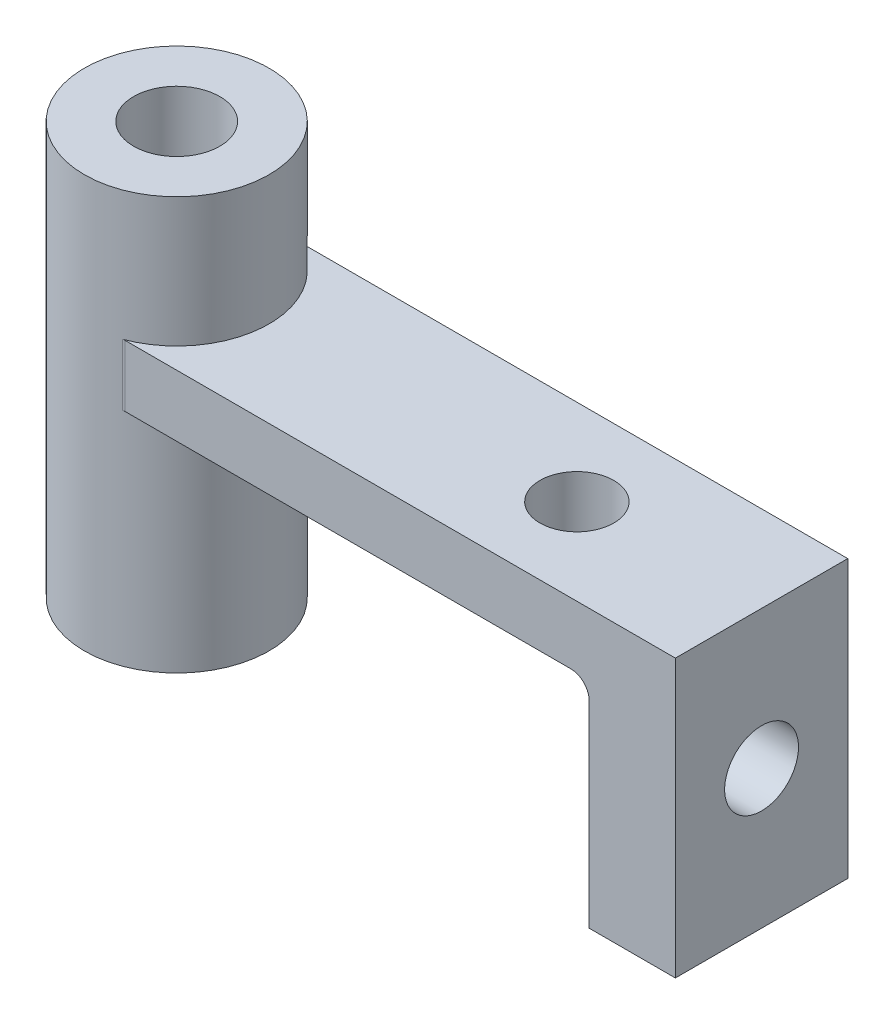
ISO-10303-21;
HEADER;
FILE_DESCRIPTION(('STEP AP214'),'2;1');
FILE_NAME('part.step','',(''),(''),'','','');
FILE_SCHEMA(('AUTOMOTIVE_DESIGN { 1 0 10303 214 1 1 1 1 }'));
ENDSEC;
DATA;
#1=APPLICATION_CONTEXT('core data for automotive mechanical design processes');
#2=APPLICATION_PROTOCOL_DEFINITION('international standard','automotive_design',2000,#1);
#3=PRODUCT_CONTEXT('',#1,'mechanical');
#4=PRODUCT('Part','Part','',(#3));
#5=PRODUCT_RELATED_PRODUCT_CATEGORY('part','',(#4));
#6=PRODUCT_DEFINITION_FORMATION('','',#4);
#7=PRODUCT_DEFINITION_CONTEXT('part definition',#1,'design');
#8=PRODUCT_DEFINITION('design','',#6,#7);
#9=PRODUCT_DEFINITION_SHAPE('','',#8);
#10=(LENGTH_UNIT() NAMED_UNIT(*) SI_UNIT(.MILLI.,.METRE.));
#11=(NAMED_UNIT(*) PLANE_ANGLE_UNIT() SI_UNIT($,.RADIAN.));
#12=(NAMED_UNIT(*) SI_UNIT($,.STERADIAN.) SOLID_ANGLE_UNIT());
#13=UNCERTAINTY_MEASURE_WITH_UNIT(LENGTH_MEASURE(1.E-05),#10,'distance_accuracy_value','');
#14=(GEOMETRIC_REPRESENTATION_CONTEXT(3) GLOBAL_UNCERTAINTY_ASSIGNED_CONTEXT((#13)) GLOBAL_UNIT_ASSIGNED_CONTEXT((#10,
#11,#12)) REPRESENTATION_CONTEXT('',''));
#15=CARTESIAN_POINT('',(0.,0.,0.));
#16=DIRECTION('',(0.,0.,1.));
#17=DIRECTION('',(1.,0.,0.));
#18=AXIS2_PLACEMENT_3D('',#15,#16,#17);
#19=CARTESIAN_POINT('',(78.,-3.,28.));
#20=DIRECTION('',(0.,0.,-1.));
#21=DIRECTION('',(-1.,0.,0.));
#22=AXIS2_PLACEMENT_3D('',#19,#20,#21);
#23=PLANE('',#22);
#24=DIRECTION('',(-1.,0.,0.));
#25=VECTOR('',#24,1.);
#26=CARTESIAN_POINT('',(95.,9.99999999999999,28.));
#27=LINE('',#26,#25);
#28=CARTESIAN_POINT('',(95.,9.99999999999999,28.));
#29=VERTEX_POINT('',#28);
#30=CARTESIAN_POINT('',(5.56776436283002,9.99999999999999,28.));
#31=VERTEX_POINT('',#30);
#32=EDGE_CURVE('E145',#29,#31,#27,.T.);
#33=ORIENTED_EDGE('',*,*,#32,.T.);
#34=DIRECTION('',(0.,1.,0.));
#35=VECTOR('',#34,1.);
#36=CARTESIAN_POINT('',(5.56776436283002,0.,28.));
#37=LINE('',#36,#35);
#38=CARTESIAN_POINT('',(5.56776436283002,0.,28.));
#39=VERTEX_POINT('',#38);
#40=EDGE_CURVE('E63',#31,#39,#37,.F.);
#41=ORIENTED_EDGE('',*,*,#40,.T.);
#42=DIRECTION('',(1.,0.,0.));
#43=VECTOR('',#42,1.);
#44=CARTESIAN_POINT('',(0.,0.,28.));
#45=LINE('',#44,#43);
#46=CARTESIAN_POINT('',(78.,0.,28.));
#47=VERTEX_POINT('',#46);
#48=EDGE_CURVE('E111',#39,#47,#45,.T.);
#49=ORIENTED_EDGE('',*,*,#48,.T.);
#50=CARTESIAN_POINT('',(78.,-3.,28.));
#51=DIRECTION('',(0.,0.,-1.));
#52=DIRECTION('',(-1.,0.,0.));
#53=AXIS2_PLACEMENT_3D('',#50,#51,#52);
#54=CIRCLE('',#53,3.);
#55=CARTESIAN_POINT('',(81.,-3.00000000000002,28.));
#56=VERTEX_POINT('',#55);
#57=EDGE_CURVE('E112',#47,#56,#54,.T.);
#58=ORIENTED_EDGE('',*,*,#57,.T.);
#59=DIRECTION('',(0.,-1.,0.));
#60=VECTOR('',#59,1.);
#61=CARTESIAN_POINT('',(81.,-3.00000000000002,28.));
#62=LINE('',#61,#60);
#63=CARTESIAN_POINT('',(81.,-35.,28.));
#64=VERTEX_POINT('',#63);
#65=EDGE_CURVE('E135',#56,#64,#62,.T.);
#66=ORIENTED_EDGE('',*,*,#65,.T.);
#67=DIRECTION('',(1.,0.,0.));
#68=VECTOR('',#67,1.);
#69=CARTESIAN_POINT('',(81.,-35.,28.));
#70=LINE('',#69,#68);
#71=CARTESIAN_POINT('',(95.,-35.,28.));
#72=VERTEX_POINT('',#71);
#73=EDGE_CURVE('E132',#64,#72,#70,.T.);
#74=ORIENTED_EDGE('',*,*,#73,.T.);
#75=DIRECTION('',(0.,1.,0.));
#76=VECTOR('',#75,1.);
#77=CARTESIAN_POINT('',(95.,-35.,28.));
#78=LINE('',#77,#76);
#79=EDGE_CURVE('E140',#72,#29,#78,.T.);
#80=ORIENTED_EDGE('',*,*,#79,.T.);
#81=EDGE_LOOP('',(#33,#41,#49,#58,#66,#74,#80));
#82=FACE_BOUND('',#81,.T.);
#83=ADVANCED_FACE('F43',(#82),#23,.F.);
#84=CARTESIAN_POINT('',(78.,-3.,0.));
#85=DIRECTION('',(0.,0.,-1.));
#86=DIRECTION('',(-1.,0.,0.));
#87=AXIS2_PLACEMENT_3D('',#84,#85,#86);
#88=PLANE('',#87);
#89=DIRECTION('',(1.,0.,0.));
#90=VECTOR('',#89,1.);
#91=CARTESIAN_POINT('',(0.,0.,0.));
#92=LINE('',#91,#90);
#93=CARTESIAN_POINT('',(5.56776436283002,0.,0.));
#94=VERTEX_POINT('',#93);
#95=CARTESIAN_POINT('',(78.,0.,0.));
#96=VERTEX_POINT('',#95);
#97=EDGE_CURVE('E121',#94,#96,#92,.T.);
#98=ORIENTED_EDGE('',*,*,#97,.F.);
#99=DIRECTION('',(0.,-1.,0.));
#100=VECTOR('',#99,1.);
#101=CARTESIAN_POINT('',(5.56776436283002,-3.,0.));
#102=LINE('',#101,#100);
#103=CARTESIAN_POINT('',(5.56776436283002,9.99999999999999,0.));
#104=VERTEX_POINT('',#103);
#105=EDGE_CURVE('E126',#94,#104,#102,.F.);
#106=ORIENTED_EDGE('',*,*,#105,.T.);
#107=DIRECTION('',(-1.,0.,0.));
#108=VECTOR('',#107,1.);
#109=CARTESIAN_POINT('',(95.,9.99999999999999,0.));
#110=LINE('',#109,#108);
#111=CARTESIAN_POINT('',(95.,9.99999999999999,0.));
#112=VERTEX_POINT('',#111);
#113=EDGE_CURVE('E117',#112,#104,#110,.T.);
#114=ORIENTED_EDGE('',*,*,#113,.F.);
#115=DIRECTION('',(0.,1.,0.));
#116=VECTOR('',#115,1.);
#117=CARTESIAN_POINT('',(95.,-35.,0.));
#118=LINE('',#117,#116);
#119=CARTESIAN_POINT('',(95.,-35.,0.));
#120=VERTEX_POINT('',#119);
#121=EDGE_CURVE('E155',#120,#112,#118,.T.);
#122=ORIENTED_EDGE('',*,*,#121,.F.);
#123=DIRECTION('',(1.,0.,0.));
#124=VECTOR('',#123,1.);
#125=CARTESIAN_POINT('',(81.,-35.,0.));
#126=LINE('',#125,#124);
#127=CARTESIAN_POINT('',(81.,-35.,0.));
#128=VERTEX_POINT('',#127);
#129=EDGE_CURVE('E154',#128,#120,#126,.T.);
#130=ORIENTED_EDGE('',*,*,#129,.F.);
#131=DIRECTION('',(0.,-1.,0.));
#132=VECTOR('',#131,1.);
#133=CARTESIAN_POINT('',(81.,-3.00000000000002,0.));
#134=LINE('',#133,#132);
#135=CARTESIAN_POINT('',(81.,-3.00000000000002,0.));
#136=VERTEX_POINT('',#135);
#137=EDGE_CURVE('E148',#136,#128,#134,.T.);
#138=ORIENTED_EDGE('',*,*,#137,.F.);
#139=CARTESIAN_POINT('',(78.,-3.,0.));
#140=DIRECTION('',(0.,0.,-1.));
#141=DIRECTION('',(-1.,0.,0.));
#142=AXIS2_PLACEMENT_3D('',#139,#140,#141);
#143=CIRCLE('',#142,3.);
#144=EDGE_CURVE('E149',#96,#136,#143,.T.);
#145=ORIENTED_EDGE('',*,*,#144,.F.);
#146=EDGE_LOOP('',(#98,#106,#114,#122,#130,#138,#145));
#147=FACE_BOUND('',#146,.T.);
#148=ADVANCED_FACE('F183',(#147),#88,.T.);
#149=CARTESIAN_POINT('',(0.,0.,28.));
#150=DIRECTION('',(0.,1.,0.));
#151=DIRECTION('',(0.,0.,1.));
#152=AXIS2_PLACEMENT_3D('',#149,#150,#151);
#153=PLANE('',#152);
#154=CARTESIAN_POINT('',(65.,0.,14.));
#155=DIRECTION('',(0.,1.,0.));
#156=DIRECTION('',(0.,0.,1.));
#157=AXIS2_PLACEMENT_3D('',#154,#155,#156);
#158=CIRCLE('',#157,6.);
#159=CARTESIAN_POINT('',(65.,0.,20.));
#160=VERTEX_POINT('',#159);
#161=EDGE_CURVE('E221',#160,#160,#158,.T.);
#162=ORIENTED_EDGE('',*,*,#161,.T.);
#163=EDGE_LOOP('',(#162));
#164=FACE_BOUND('',#163,.T.);
#165=CARTESIAN_POINT('',(0.,0.,14.));
#166=DIRECTION('',(0.,1.,0.));
#167=DIRECTION('',(0.,0.,1.));
#168=AXIS2_PLACEMENT_3D('',#165,#166,#167);
#169=CIRCLE('',#168,15.);
#170=CARTESIAN_POINT('',(5.21977909015315,0.,-0.0624999999999983));
#171=VERTEX_POINT('',#170);
#172=CARTESIAN_POINT('',(5.21977909015314,0.,28.0625));
#173=VERTEX_POINT('',#172);
#174=EDGE_CURVE('E146',#171,#173,#169,.F.);
#175=ORIENTED_EDGE('',*,*,#174,.F.);
#176=CARTESIAN_POINT('',(5.56776436283002,0.,-0.999999999999999));
#177=DIRECTION('',(0.,1.,0.));
#178=DIRECTION('',(0.,0.,1.));
#179=AXIS2_PLACEMENT_3D('',#176,#177,#178);
#180=CIRCLE('',#179,1.);
#181=EDGE_CURVE('E178',#171,#94,#180,.T.);
#182=ORIENTED_EDGE('',*,*,#181,.T.);
#183=ORIENTED_EDGE('',*,*,#97,.T.);
#184=DIRECTION('',(0.,0.,-1.));
#185=VECTOR('',#184,1.);
#186=CARTESIAN_POINT('',(78.,0.,28.));
#187=LINE('',#186,#185);
#188=EDGE_CURVE('E122',#47,#96,#187,.T.);
#189=ORIENTED_EDGE('',*,*,#188,.F.);
#190=ORIENTED_EDGE('',*,*,#48,.F.);
#191=CARTESIAN_POINT('',(5.56776436283002,0.,29.));
#192=DIRECTION('',(0.,1.,0.));
#193=DIRECTION('',(0.,0.,1.));
#194=AXIS2_PLACEMENT_3D('',#191,#192,#193);
#195=CIRCLE('',#194,1.);
#196=EDGE_CURVE('E11',#39,#173,#195,.T.);
#197=ORIENTED_EDGE('',*,*,#196,.T.);
#198=EDGE_LOOP('',(#175,#182,#183,#189,#190,#197));
#199=FACE_BOUND('',#198,.T.);
#200=ADVANCED_FACE('F125',(#164,#199),#153,.F.);
#201=CARTESIAN_POINT('',(78.,-3.,28.));
#202=DIRECTION('',(0.,0.,-1.));
#203=DIRECTION('',(-1.,0.,0.));
#204=AXIS2_PLACEMENT_3D('',#201,#202,#203);
#205=CYLINDRICAL_SURFACE('',#204,3.);
#206=ORIENTED_EDGE('',*,*,#144,.T.);
#207=DIRECTION('',(0.,0.,-1.));
#208=VECTOR('',#207,1.);
#209=CARTESIAN_POINT('',(81.,-3.00000000000002,28.));
#210=LINE('',#209,#208);
#211=EDGE_CURVE('E130',#56,#136,#210,.T.);
#212=ORIENTED_EDGE('',*,*,#211,.F.);
#213=ORIENTED_EDGE('',*,*,#57,.F.);
#214=ORIENTED_EDGE('',*,*,#188,.T.);
#215=EDGE_LOOP('',(#206,#212,#213,#214));
#216=FACE_BOUND('',#215,.T.);
#217=ADVANCED_FACE('F127',(#216),#205,.F.);
#218=CARTESIAN_POINT('',(81.,-3.00000000000002,28.));
#219=DIRECTION('',(1.,0.,0.));
#220=DIRECTION('',(0.,0.,-1.));
#221=AXIS2_PLACEMENT_3D('',#218,#219,#220);
#222=PLANE('',#221);
#223=CARTESIAN_POINT('',(81.,-12.5,14.));
#224=DIRECTION('',(1.,0.,0.));
#225=DIRECTION('',(0.,0.,-1.));
#226=AXIS2_PLACEMENT_3D('',#223,#224,#225);
#227=CIRCLE('',#226,6.);
#228=CARTESIAN_POINT('',(81.,-12.5,8.));
#229=VERTEX_POINT('',#228);
#230=EDGE_CURVE('E227',#229,#229,#227,.T.);
#231=ORIENTED_EDGE('',*,*,#230,.T.);
#232=EDGE_LOOP('',(#231));
#233=FACE_BOUND('',#232,.T.);
#234=ORIENTED_EDGE('',*,*,#137,.T.);
#235=DIRECTION('',(0.,0.,-1.));
#236=VECTOR('',#235,1.);
#237=CARTESIAN_POINT('',(81.,-35.,28.));
#238=LINE('',#237,#236);
#239=EDGE_CURVE('E162',#64,#128,#238,.T.);
#240=ORIENTED_EDGE('',*,*,#239,.F.);
#241=ORIENTED_EDGE('',*,*,#65,.F.);
#242=ORIENTED_EDGE('',*,*,#211,.T.);
#243=EDGE_LOOP('',(#234,#240,#241,#242));
#244=FACE_BOUND('',#243,.T.);
#245=ADVANCED_FACE('F202',(#233,#244),#222,.F.);
#246=CARTESIAN_POINT('',(81.,-35.,28.));
#247=DIRECTION('',(0.,1.,0.));
#248=DIRECTION('',(0.,0.,1.));
#249=AXIS2_PLACEMENT_3D('',#246,#247,#248);
#250=PLANE('',#249);
#251=ORIENTED_EDGE('',*,*,#129,.T.);
#252=DIRECTION('',(0.,0.,-1.));
#253=VECTOR('',#252,1.);
#254=CARTESIAN_POINT('',(95.,-35.,28.));
#255=LINE('',#254,#253);
#256=EDGE_CURVE('E158',#72,#120,#255,.T.);
#257=ORIENTED_EDGE('',*,*,#256,.F.);
#258=ORIENTED_EDGE('',*,*,#73,.F.);
#259=ORIENTED_EDGE('',*,*,#239,.T.);
#260=EDGE_LOOP('',(#251,#257,#258,#259));
#261=FACE_BOUND('',#260,.T.);
#262=ADVANCED_FACE('F198',(#261),#250,.F.);
#263=CARTESIAN_POINT('',(95.,-35.,28.));
#264=DIRECTION('',(-1.,0.,0.));
#265=DIRECTION('',(0.,0.,1.));
#266=AXIS2_PLACEMENT_3D('',#263,#264,#265);
#267=PLANE('',#266);
#268=CARTESIAN_POINT('',(95.,-12.5,14.));
#269=DIRECTION('',(1.,0.,0.));
#270=DIRECTION('',(0.,0.,-1.));
#271=AXIS2_PLACEMENT_3D('',#268,#269,#270);
#272=CIRCLE('',#271,6.);
#273=CARTESIAN_POINT('',(95.,-12.5,8.));
#274=VERTEX_POINT('',#273);
#275=EDGE_CURVE('E229',#274,#274,#272,.T.);
#276=ORIENTED_EDGE('',*,*,#275,.F.);
#277=EDGE_LOOP('',(#276));
#278=FACE_BOUND('',#277,.T.);
#279=ORIENTED_EDGE('',*,*,#121,.T.);
#280=DIRECTION('',(0.,0.,-1.));
#281=VECTOR('',#280,1.);
#282=CARTESIAN_POINT('',(95.,9.99999999999999,28.));
#283=LINE('',#282,#281);
#284=EDGE_CURVE('E144',#29,#112,#283,.T.);
#285=ORIENTED_EDGE('',*,*,#284,.F.);
#286=ORIENTED_EDGE('',*,*,#79,.F.);
#287=ORIENTED_EDGE('',*,*,#256,.T.);
#288=EDGE_LOOP('',(#279,#285,#286,#287));
#289=FACE_BOUND('',#288,.T.);
#290=ADVANCED_FACE('F193',(#278,#289),#267,.F.);
#291=CARTESIAN_POINT('',(95.,9.99999999999999,28.));
#292=DIRECTION('',(0.,-1.,0.));
#293=DIRECTION('',(0.,0.,-1.));
#294=AXIS2_PLACEMENT_3D('',#291,#292,#293);
#295=PLANE('',#294);
#296=CARTESIAN_POINT('',(65.,9.99999999999999,14.));
#297=DIRECTION('',(0.,1.,0.));
#298=DIRECTION('',(0.,0.,1.));
#299=AXIS2_PLACEMENT_3D('',#296,#297,#298);
#300=CIRCLE('',#299,6.);
#301=CARTESIAN_POINT('',(65.,9.99999999999999,20.));
#302=VERTEX_POINT('',#301);
#303=EDGE_CURVE('E223',#302,#302,#300,.T.);
#304=ORIENTED_EDGE('',*,*,#303,.F.);
#305=EDGE_LOOP('',(#304));
#306=FACE_BOUND('',#305,.T.);
#307=CARTESIAN_POINT('',(0.,9.99999999999999,14.));
#308=DIRECTION('',(0.,-1.,0.));
#309=DIRECTION('',(0.,0.,-1.));
#310=AXIS2_PLACEMENT_3D('',#307,#308,#309);
#311=CIRCLE('',#310,15.);
#312=CARTESIAN_POINT('',(5.21977909015314,9.99999999999999,28.0625));
#313=VERTEX_POINT('',#312);
#314=CARTESIAN_POINT('',(5.21977909015315,9.99999999999999,-0.0624999999999986));
#315=VERTEX_POINT('',#314);
#316=EDGE_CURVE('E186',#313,#315,#311,.F.);
#317=ORIENTED_EDGE('',*,*,#316,.F.);
#318=CARTESIAN_POINT('',(5.56776436283002,9.99999999999999,29.));
#319=DIRECTION('',(0.,-1.,0.));
#320=DIRECTION('',(0.,0.,-1.));
#321=AXIS2_PLACEMENT_3D('',#318,#319,#320);
#322=CIRCLE('',#321,1.);
#323=EDGE_CURVE('E51',#313,#31,#322,.T.);
#324=ORIENTED_EDGE('',*,*,#323,.T.);
#325=ORIENTED_EDGE('',*,*,#32,.F.);
#326=ORIENTED_EDGE('',*,*,#284,.T.);
#327=ORIENTED_EDGE('',*,*,#113,.T.);
#328=CARTESIAN_POINT('',(5.56776436283002,9.99999999999999,-0.999999999999999));
#329=DIRECTION('',(0.,-1.,0.));
#330=DIRECTION('',(0.,0.,-1.));
#331=AXIS2_PLACEMENT_3D('',#328,#329,#330);
#332=CIRCLE('',#331,1.);
#333=EDGE_CURVE('E174',#104,#315,#332,.T.);
#334=ORIENTED_EDGE('',*,*,#333,.T.);
#335=EDGE_LOOP('',(#317,#324,#325,#326,#327,#334));
#336=FACE_BOUND('',#335,.T.);
#337=ADVANCED_FACE('F189',(#306,#336),#295,.F.);
#338=CARTESIAN_POINT('',(0.,31.,14.));
#339=DIRECTION('',(0.,-1.,0.));
#340=DIRECTION('',(0.,0.,-1.));
#341=AXIS2_PLACEMENT_3D('',#338,#339,#340);
#342=CYLINDRICAL_SURFACE('',#341,7.);
#343=CARTESIAN_POINT('',(0.,31.,14.));
#344=DIRECTION('',(0.,1.,0.));
#345=DIRECTION('',(0.,0.,1.));
#346=AXIS2_PLACEMENT_3D('',#343,#344,#345);
#347=CIRCLE('',#346,7.);
#348=CARTESIAN_POINT('',(0.,31.,21.));
#349=VERTEX_POINT('',#348);
#350=EDGE_CURVE('E211',#349,#349,#347,.T.);
#351=ORIENTED_EDGE('',*,*,#350,.T.);
#352=EDGE_LOOP('',(#351));
#353=FACE_BOUND('',#352,.T.);
#354=CARTESIAN_POINT('',(0.,-36.,14.));
#355=DIRECTION('',(0.,1.,0.));
#356=DIRECTION('',(0.,0.,1.));
#357=AXIS2_PLACEMENT_3D('',#354,#355,#356);
#358=CIRCLE('',#357,7.);
#359=CARTESIAN_POINT('',(0.,-36.,21.));
#360=VERTEX_POINT('',#359);
#361=EDGE_CURVE('E220',#360,#360,#358,.T.);
#362=ORIENTED_EDGE('',*,*,#361,.F.);
#363=EDGE_LOOP('',(#362));
#364=FACE_BOUND('',#363,.T.);
#365=ADVANCED_FACE('F243',(#353,#364),#342,.F.);
#366=CARTESIAN_POINT('',(0.,31.,14.));
#367=DIRECTION('',(0.,-1.,0.));
#368=DIRECTION('',(0.,0.,-1.));
#369=AXIS2_PLACEMENT_3D('',#366,#367,#368);
#370=CYLINDRICAL_SURFACE('',#369,15.);
#371=CARTESIAN_POINT('',(0.,31.,14.));
#372=DIRECTION('',(0.,1.,0.));
#373=DIRECTION('',(0.,0.,1.));
#374=AXIS2_PLACEMENT_3D('',#371,#372,#373);
#375=CIRCLE('',#374,15.);
#376=CARTESIAN_POINT('',(0.,31.,29.));
#377=VERTEX_POINT('',#376);
#378=EDGE_CURVE('E210',#377,#377,#375,.T.);
#379=ORIENTED_EDGE('',*,*,#378,.F.);
#380=EDGE_LOOP('',(#379));
#381=FACE_BOUND('',#380,.T.);
#382=CARTESIAN_POINT('',(0.,-36.,14.));
#383=DIRECTION('',(0.,1.,0.));
#384=DIRECTION('',(0.,0.,1.));
#385=AXIS2_PLACEMENT_3D('',#382,#383,#384);
#386=CIRCLE('',#385,15.);
#387=CARTESIAN_POINT('',(0.,-36.,29.));
#388=VERTEX_POINT('',#387);
#389=EDGE_CURVE('E212',#388,#388,#386,.T.);
#390=ORIENTED_EDGE('',*,*,#389,.T.);
#391=EDGE_LOOP('',(#390));
#392=FACE_BOUND('',#391,.T.);
#393=ORIENTED_EDGE('',*,*,#316,.T.);
#394=DIRECTION('',(0.,-1.,0.));
#395=VECTOR('',#394,1.);
#396=CARTESIAN_POINT('',(5.21977909015315,31.,-0.0624999999999983));
#397=LINE('',#396,#395);
#398=EDGE_CURVE('E171',#315,#171,#397,.T.);
#399=ORIENTED_EDGE('',*,*,#398,.T.);
#400=ORIENTED_EDGE('',*,*,#174,.T.);
#401=DIRECTION('',(0.,-1.,0.));
#402=VECTOR('',#401,1.);
#403=CARTESIAN_POINT('',(5.21977909015314,31.,28.0625));
#404=LINE('',#403,#402);
#405=EDGE_CURVE('E166',#173,#313,#404,.F.);
#406=ORIENTED_EDGE('',*,*,#405,.T.);
#407=EDGE_LOOP('',(#393,#399,#400,#406));
#408=FACE_BOUND('',#407,.T.);
#409=ADVANCED_FACE('F207',(#381,#392,#408),#370,.T.);
#410=CARTESIAN_POINT('',(0.,31.,14.));
#411=DIRECTION('',(0.,1.,0.));
#412=DIRECTION('',(0.,0.,1.));
#413=AXIS2_PLACEMENT_3D('',#410,#411,#412);
#414=PLANE('',#413);
#415=ORIENTED_EDGE('',*,*,#378,.T.);
#416=EDGE_LOOP('',(#415));
#417=FACE_BOUND('',#416,.T.);
#418=ORIENTED_EDGE('',*,*,#350,.F.);
#419=EDGE_LOOP('',(#418));
#420=FACE_BOUND('',#419,.T.);
#421=ADVANCED_FACE('F259',(#417,#420),#414,.T.);
#422=CARTESIAN_POINT('',(0.,-36.,14.));
#423=DIRECTION('',(0.,1.,0.));
#424=DIRECTION('',(0.,0.,1.));
#425=AXIS2_PLACEMENT_3D('',#422,#423,#424);
#426=PLANE('',#425);
#427=ORIENTED_EDGE('',*,*,#361,.T.);
#428=EDGE_LOOP('',(#427));
#429=FACE_BOUND('',#428,.T.);
#430=ORIENTED_EDGE('',*,*,#389,.F.);
#431=EDGE_LOOP('',(#430));
#432=FACE_BOUND('',#431,.T.);
#433=ADVANCED_FACE('F257',(#429,#432),#426,.F.);
#434=CARTESIAN_POINT('',(5.56776436283002,31.,-0.999999999999999));
#435=DIRECTION('',(0.,-1.,0.));
#436=DIRECTION('',(0.,0.,-1.));
#437=AXIS2_PLACEMENT_3D('',#434,#435,#436);
#438=CYLINDRICAL_SURFACE('',#437,1.);
#439=ORIENTED_EDGE('',*,*,#181,.F.);
#440=ORIENTED_EDGE('',*,*,#398,.F.);
#441=ORIENTED_EDGE('',*,*,#333,.F.);
#442=ORIENTED_EDGE('',*,*,#105,.F.);
#443=EDGE_LOOP('',(#439,#440,#441,#442));
#444=FACE_BOUND('',#443,.T.);
#445=ADVANCED_FACE('F190',(#444),#438,.F.);
#446=CARTESIAN_POINT('',(5.56776436283002,31.,29.));
#447=DIRECTION('',(0.,-1.,0.));
#448=DIRECTION('',(0.,0.,-1.));
#449=AXIS2_PLACEMENT_3D('',#446,#447,#448);
#450=CYLINDRICAL_SURFACE('',#449,1.);
#451=ORIENTED_EDGE('',*,*,#196,.F.);
#452=ORIENTED_EDGE('',*,*,#40,.F.);
#453=ORIENTED_EDGE('',*,*,#323,.F.);
#454=ORIENTED_EDGE('',*,*,#405,.F.);
#455=EDGE_LOOP('',(#451,#452,#453,#454));
#456=FACE_BOUND('',#455,.T.);
#457=ADVANCED_FACE('F44',(#456),#450,.F.);
#458=CARTESIAN_POINT('',(65.,-122.,14.));
#459=DIRECTION('',(0.,1.,0.));
#460=DIRECTION('',(0.,0.,1.));
#461=AXIS2_PLACEMENT_3D('',#458,#459,#460);
#462=CYLINDRICAL_SURFACE('',#461,6.);
#463=ORIENTED_EDGE('',*,*,#303,.T.);
#464=EDGE_LOOP('',(#463));
#465=FACE_BOUND('',#464,.T.);
#466=ORIENTED_EDGE('',*,*,#161,.F.);
#467=EDGE_LOOP('',(#466));
#468=FACE_BOUND('',#467,.T.);
#469=ADVANCED_FACE('F269',(#465,#468),#462,.F.);
#470=CARTESIAN_POINT('',(53.,-12.5,14.));
#471=DIRECTION('',(1.,0.,0.));
#472=DIRECTION('',(0.,0.,-1.));
#473=AXIS2_PLACEMENT_3D('',#470,#471,#472);
#474=CYLINDRICAL_SURFACE('',#473,6.);
#475=ORIENTED_EDGE('',*,*,#275,.T.);
#476=EDGE_LOOP('',(#475));
#477=FACE_BOUND('',#476,.T.);
#478=ORIENTED_EDGE('',*,*,#230,.F.);
#479=EDGE_LOOP('',(#478));
#480=FACE_BOUND('',#479,.T.);
#481=ADVANCED_FACE('F234',(#477,#480),#474,.F.);
#482=CLOSED_SHELL('',(#83,#148,#200,#217,#245,#262,#290,#337,#365,#409,#421,#433,#445,#457,#469,#481));
#483=MANIFOLD_SOLID_BREP('B2',#482);
#484=ADVANCED_BREP_SHAPE_REPRESENTATION('',(#18,#483),#14);
#485=SHAPE_DEFINITION_REPRESENTATION(#9,#484);
ENDSEC;
END-ISO-10303-21;
